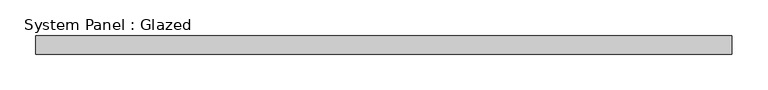
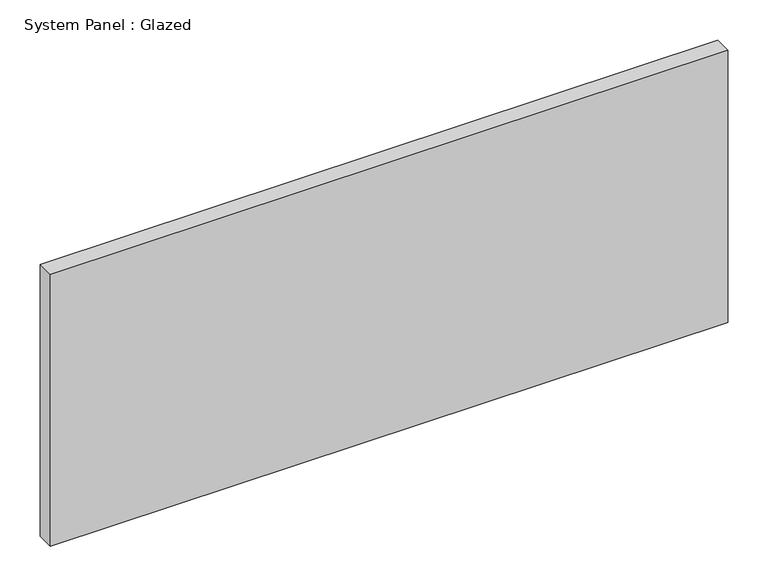
"""IFC4 building model written with IfcOpenShell, lengths in millimetres: plate geometry, System Panel : Glazed."""

from ifc_helpers import new_model, si_unit, origin, origin_with_axes, place, context, project, spatial, polyline, outline, extrude, source, transform, mapped, element, save


def system_panel_glazed_06453807(model_context):
    return source(origin(), model_context, "Body", "SweptSolid", [
        extrude(outline(polyline([(485.775, 19.05), (-485.775, 19.05), (-485.775, 44.45), (485.775, 44.45), (485.775, 19.05)])), origin_with_axes(), (0.0, 0.0, 1.0), 412.75),
    ])


if __name__ == "__main__":
    model = new_model("IFC4")
    model_context = context("Model", 3, world=origin())
    ifc_project = project(units=[si_unit("LENGTHUNIT", "METRE", prefix="MILLI")], contexts=[model_context])
    site = spatial("IfcSite", under=ifc_project)
    building = spatial("IfcBuilding", under=site)
    placement = place(None, origin())
    system_panel_glazed_shape = system_panel_glazed_06453807(model_context)
    element("IfcPlate", 1, ObjectType="System Panel : Glazed", at=placement, inside=building, context=model_context, shape_type="MappedRepresentation", body=[
        mapped(system_panel_glazed_shape, transform((0.0, 0.0, 0.0), x_axis=(1.0, 0.0, 0.0), y_axis=(0.0, 1.0, 0.0), z_axis=(0.0, 0.0, 1.0))),
    ])
    save(model, "model.ifc")

# Revit data of these elements
# Type "System Panel : Glazed"
#   Construction Type Id = "GSP4R"
#   Analytic Construction = "1/8 in Pilkington single glazing"
#   Visual Light Transmittance = 0.9
#   Solar Heat Gain Coefficient = 0.86
#   Heat Transfer Coefficient (U) = 1.18115 BTU/(h·ft²·°F)
#   Define Thermal Properties by = 1
# Element 1 (IfcPlate, "System Panel : Glazed")
#   Materials on its faces: "Glass"
# Materials
#   "Glass": class "Glass", colour RGB 0 128 192, transparency 0.75, Description = "Soda Lime Glass", Cost = 0
